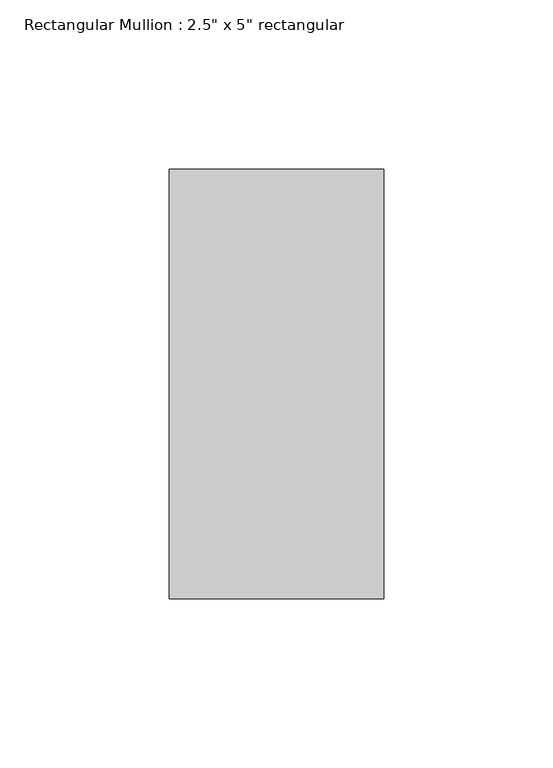
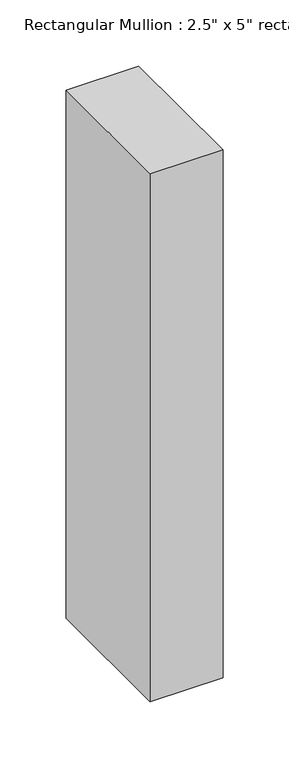
"""IFC4 building model written with IfcOpenShell, lengths in millimetres: member geometry."""

from ifc_helpers import new_model, si_unit, frame, origin, place, context, project, spatial, polyline, outline, extrude, source, transform, mapped, element, save


def member_d55fe2b3(model_context):
    return source(origin(), model_context, "Body", "SweptSolid", [
        extrude(outline(polyline([(0.0, 63.5), (0.0, -63.5), (-63.5, -63.5), (-63.5, 63.5), (0.0, 63.5)])), frame((0.0, 0.0, -487.0221123), z_axis=(0.0, 0.0, 1.0), x_axis=(1.0, 0.0, 0.0)), (0.0, 0.0, 1.0), 487.0221123),
    ])


if __name__ == "__main__":
    model = new_model("IFC4")
    model_context = context("Model", 3, world=origin())
    ifc_project = project(units=[si_unit("LENGTHUNIT", "METRE", prefix="MILLI")], contexts=[model_context])
    site = spatial("IfcSite", under=ifc_project)
    building = spatial("IfcBuilding", under=site)
    placement = place(None, origin())
    member_shape = member_d55fe2b3(model_context)
    element("IfcMember", 1, ObjectType="Rectangular Mullion : 2.5\" x 5\" rectangular", at=placement, inside=building, context=model_context, shape_type="MappedRepresentation", body=[
        mapped(member_shape, transform((0.0, 0.0, 0.0), x_axis=(1.0, 0.0, 0.0), y_axis=(0.0, 1.0, 0.0), z_axis=(0.0, 0.0, 1.0))),
    ])
    save(model, "model.ifc")

# Revit data of these elements
# Type "Rectangular Mullion : 2.5\" x 5\" rectangular"
#   built-in parameter 1007304 = 0.416667 (stored number, unit not read)
#   built-in parameter 1007301 = 0.104167 (stored number, unit not read)
#   built-in parameter 1007300 = 0.104167 (stored number, unit not read)
# Element 1 (IfcMember, "Rectangular Mullion : 2.5\" x 5\" rectangular")
#   Materials on its faces: "Aluminum"
# Materials
#   "Aluminum": class "Metal", colour RGB 247 247 247, transparency 0, Description = "Aluminum 6061", Cost = 0
